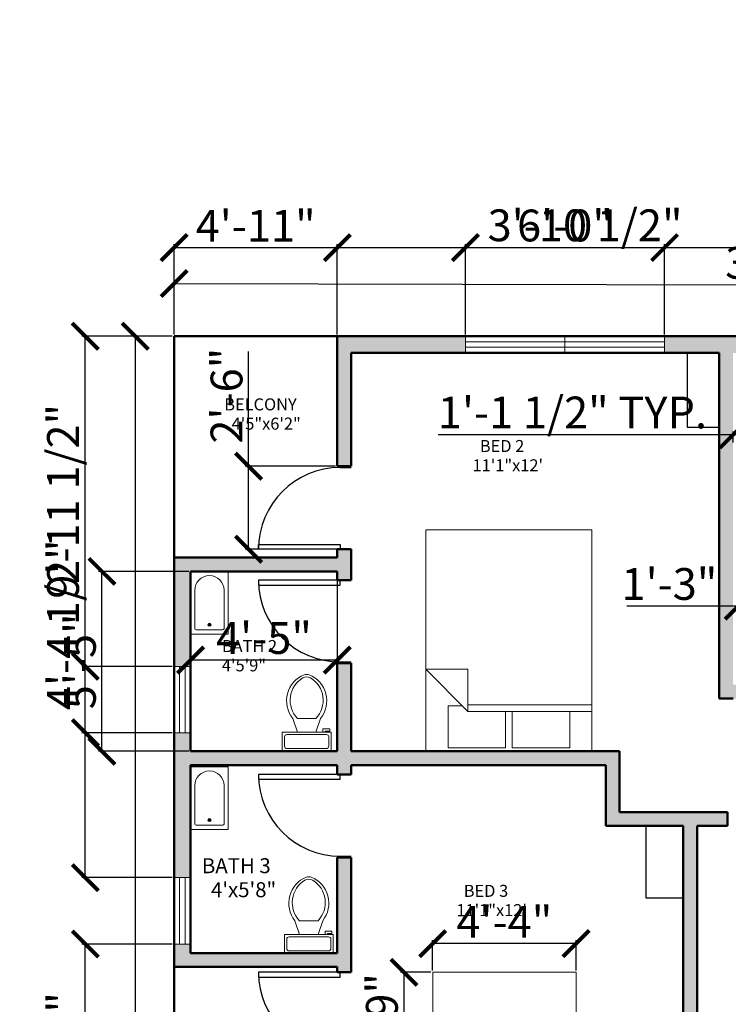
# Model space of a CAD drawing. Units: inches. Extents: x 3147 to 3847, y 1414 to 2207.
# Tile 6 of 7: x 3294 to 3550, y 1852 to 2207. Entities that reach past the tile are written whole.
import ezdxf

# ---------------------------------------------------------------- set-up
doc = ezdxf.new("R2010")
doc.units = ezdxf.units.IN
for name, color, linetype, lineweight in [('A-ANNO-DIMS', 2, 'Continuous', 18), ('A-AREA-IDEN', 7, 'Continuous', 18), ('A-DOOR', 3, 'Continuous', 25), ('A-FLOR-CASE', 32, 'Continuous', 25), ('A-FLOR-FIXT', 9, 'Continuous', 18), ('A-FURN', 8, 'Continuous', 18), ('A-GLAZ', 4, 'Continuous', 18), ('A-WALL', 7, 'Continuous', 50)]:
    doc.layers.add(name, color=color, linetype=linetype, lineweight=lineweight)
doc.layers.add('A-WALL-PATT', color=18, linetype='Continuous', lineweight=13, true_color=0x000000)
doc.styles.get("Standard").update_dxf_attribs({"font": 'arial.ttf'})
doc.dimstyles.new('ISO-25', dxfattribs={"dimtxt": 11.5, "dimasz": 9.5, "dimexe": 1.25, "dimexo": 0.625, "dimtad": 1, "dimdec": 0, "dimlunit": 3, "dimtxsty": 'Standard', "dimblk": 'ARCHTICK', "dimcen": 2.5, "dimadec": 0, "dimazin": 0, "dimtfac": 1, "dimtdec": 0, "dimtmove": 0, "dimatfit": 3, "dimfxl": 1, "dimarcsym": 0})

# ---------------------------------------------------------------- blocks, each defined once
blk = doc.blocks.new('*U4')
for p, q in [((-750, 0), (-750, -100)), ((0, 0), (0, -100))]:
    blk.add_line(p, q)
blk.add_lwpolyline([(0, 0), (0, 750), (-43.75, 750), (-43.75, 0)], close=True)
blk.add_arc((0, 0), 750, 90, 180)
blk = doc.blocks.new('*U3')
for p, q in [((0, 0), (0, -100)), ((750, 0), (750, -100))]:
    blk.add_line(p, q)
blk.add_lwpolyline([(0, 0), (0, 750), (43.75, 750), (43.75, 0)], close=True)
blk.add_arc((0, 0), 750, 0, 90)
blk = doc.blocks.new('Bath Tub - 26 x 60 in.')
for p, q in [((8, -18), (10, -18)), ((9, -17), (9, -19))]:
    blk.add_line(p, q)
blk.add_lwpolyline([(0, -36), (0, 0), (60, 0), (60, -36)], close=True)
for points in [[(4, -30), (4, -6)], [(6, -4), (42, -4)], [(42, -32), (6, -32)]]:
    blk.add_lwpolyline(points)
for radius in [1.5, 1]:
    blk.add_circle((9, -18), radius)
for centre, radius, start, end in [((5.75, -5.75), 1.77, 81.8699, 188.1301), ((42, -18), 14, 270, 90), ((5.75, -30.25), 1.77, 171.8699, 278.1301)]:
    blk.add_arc(centre, radius, start, end)
blk = doc.blocks.new('Toilet - top')
for p, q in [((9.5, -6), (9.5, -2)), ((-10, -8.5), (-8, -8.5)), ((-10, -9.5), (-10, -8.5)), ((-8, -8.5), (-8, -8)), ((-7, -8), (-7, -9.5)), ((-4, -8), (-6, -14)), ((4, -8), (6, -14)), ((-7, -9.5), (-10, -9.5)), ((4, -14), (-4, -14))]:
    blk.add_line(p, q)
blk.add_lwpolyline([(10.5, -8), (10.5, 0), (-10.5, 0), (-10.5, -8)], close=True)
for points in [[(-9.5, -2), (-9.5, -6)], [(8.5, -1), (-8.5, -1)], [(-8.5, -7), (8.5, -7)]]:
    blk.add_lwpolyline(points)
for centre, radius, start, end in [((-8.62, -1.88), 0.884, 81.8699, 188.1301), ((8.62, -1.88), 0.884, 351.8699, 98.1301), ((-8.62, -6.12), 0.884, 171.8699, 278.1301), ((8.62, -6.12), 0.884, 261.8699, 8.1301), ((3.52, -21.58), 12.17, 141.4691, 247.9714), ((4.2, -21.82), 11.33, 136.3677, 238.9468), ((-3.52, -21.58), 12.17, 292.0284, 38.5307), ((-4.2, -21.82), 11.33, 301.053, 43.6321), ((0, -27.88), 4, 245.7318, 294.2682), ((0, -29), 4, 254.8605, 285.1395)]:
    blk.add_arc(centre, radius, start, end)
blk = doc.blocks.new('Bed - Queen')
for p, q in [((0, -80.00003), (0, 0)), ((0, 0), (59.99999, 0)), ((59.99999, 0), (59.99999, -80.00003)), ((7.99999, -1.2), (28.79998, -1.2)), ((7.99999, -14.4), (7.99999, -1.2)), ((28.79998, -1.2), (28.79998, -14.4)), ((31.19999, -1.2), (51.99999, -1.2)), ((31.19999, -14.4), (31.19999, -1.2)), ((51.99999, -1.2), (51.99999, -16.4)), ((0, -14.4), (44.8, -14.4)), ((44.8, -16.8), (0, -16.8)), ((59.99999, -29.6), (44.8, -14.4)), ((44.8, -14.4), (44.8, -29.6)), ((51.99999, -16.4), (46.79936, -16.4)), ((44.8, -29.6), (59.99999, -29.6)), ((59.99999, -80.00003), (0, -80.00003))]:
    blk.add_line(p, q)
blk = doc.blocks.new('_ArchTick')
at = {"color": 0, "linetype": 'ByBlock', "const_width": 0.15}
blk.add_lwpolyline([(-0.5, -0.5), (0.5, 0.5)], dxfattribs=at)
blk = doc.blocks.new('*D22')
at = {"layer": 'A-ANNO-DIMS', "color": 0, "lineweight": -2, "transparency": 16777216}
for p, q in [((3349.14, 2093.05), (3334.5, 2093.05)), ((3335.75, 2093.05), (3335.75, 1495.05)), ((3349.14, 1495.05), (3334.5, 1495.05))]:
    blk.add_line(p, q, dxfattribs=at)
at = {"layer": 'Defpoints', "color": 0, "transparency": 16777216}
for p in [(3349.76, 2093.05), (3335.75, 1495.05), (3349.76, 1495.05)]:
    blk.add_point(p, dxfattribs=at)
at = {"layer": 'A-ANNO-DIMS', "color": 0, "lineweight": -2, "transparency": 16777216, "xscale": 9.5, "yscale": 9.5, "zscale": 9.5}
for p, rotation in [((3335.75, 2093.05), 90), ((3335.75, 1495.05), 270)]:
    blk.add_blockref('_ArchTick', p, dxfattribs=dict(at, rotation=rotation))
at = {"layer": 'A-ANNO-DIMS', "color": 0, "transparency": 16777216, "insert": (3329.25, 1794.05), "char_height": 11.5, "attachment_point": 5, "rotation": 90}
blk.add_mtext('49\'-10"', dxfattribs=at)
blk = doc.blocks.new('*D23')
at = {"layer": 'A-ANNO-DIMS', "color": 0, "lineweight": -2, "transparency": 16777216}
for p, q in [((3349.77, 2094.75), (3349.81, 2113.37)), ((3349.81, 2112.12), (3769.81, 2111.04)), ((3769.77, 2093.67), (3769.81, 2112.29))]:
    blk.add_line(p, q, dxfattribs=at)
at = {"layer": 'Defpoints', "color": 0, "transparency": 16777216}
for p in [(3769.81, 2111.04), (3349.76, 2094.13), (3769.76, 2093.05)]:
    blk.add_point(p, dxfattribs=at)
at = {"layer": 'A-ANNO-DIMS', "color": 0, "lineweight": -2, "transparency": 16777216, "xscale": 9.5, "yscale": 9.5, "zscale": 9.5}
for p, rotation in [((3349.81, 2112.12), 179.8528346034433), ((3769.81, 2111.04), 359.8528346034433)]:
    blk.add_blockref('_ArchTick', p, dxfattribs=dict(at, rotation=rotation))
at = {"layer": 'A-ANNO-DIMS', "color": 0, "transparency": 16777216, "insert": (3559.83, 2118.08), "char_height": 11.5, "attachment_point": 5, "rotation": 359.8528}
blk.add_mtext("35'", dxfattribs=at)
blk = doc.blocks.new('WIN-24IN')
for p, q in [((6, 24), (0, 24)), ((2, 0), (2, 24)), ((4, 0), (4, 24)), ((6, 0), (0, 0))]:
    blk.add_line(p, q)
blk = doc.blocks.new('*D29')
at = {"layer": 'A-ANNO-DIMS', "color": 0, "lineweight": -2, "transparency": 16777216}
for p, q in [((3568.76, 2054.03), (3568.76, 2207.49)), ((3565.99, 2054.03), (3570.01, 2054.03)), ((3568.76, 2031.36), (3568.76, 2054.03)), ((3565.99, 2031.36), (3570.01, 2031.36))]:
    blk.add_line(p, q, dxfattribs=at)
at = {"layer": 'Defpoints', "color": 0, "transparency": 16777216}
for p in [(3565.36, 2054.03), (3568.76, 2054.03), (3565.36, 2031.36)]:
    blk.add_point(p, dxfattribs=at)
at = {"layer": 'A-ANNO-DIMS', "color": 0, "lineweight": -2, "transparency": 16777216, "xscale": 9.5, "yscale": 9.5, "zscale": 9.5}
for p, rotation in [((3568.76, 2054.03), 90), ((3568.76, 2031.36), 270)]:
    blk.add_blockref('_ArchTick', p, dxfattribs=dict(at, rotation=rotation))
at = {"layer": 'A-ANNO-DIMS', "color": 0, "transparency": 16777216, "insert": (3562.19, 2135.51), "char_height": 11.5, "attachment_point": 5, "rotation": 90}
blk.add_mtext('TUB 1\'-10 1/2" TYP.', dxfattribs=at)
blk = doc.blocks.new('*D30')
at = {"layer": 'A-ANNO-DIMS', "color": 0, "lineweight": -2, "transparency": 16777216}
for p, q in [((3551.76, 2057.43), (3445.2, 2057.43)), ((3551.76, 2054.65), (3551.76, 2058.68)), ((3565.36, 2057.43), (3551.76, 2057.43)), ((3565.36, 2054.65), (3565.36, 2058.68))]:
    blk.add_line(p, q, dxfattribs=at)
at = {"layer": 'Defpoints', "color": 0, "transparency": 16777216}
for p in [(3551.76, 2057.43), (3551.76, 2054.03), (3565.36, 2054.03)]:
    blk.add_point(p, dxfattribs=at)
at = {"layer": 'A-ANNO-DIMS', "color": 0, "lineweight": -2, "transparency": 16777216, "xscale": 9.5, "yscale": 9.5, "zscale": 9.5, "rotation": 180}
blk.add_blockref('_ArchTick', (3551.76, 2057.43), dxfattribs=at)
at = {"layer": 'A-ANNO-DIMS', "color": 0, "lineweight": -2, "transparency": 16777216, "xscale": 9.5, "yscale": 9.5, "zscale": 9.5}
blk.add_blockref('_ArchTick', (3565.36, 2057.43), dxfattribs=at)
at = {"layer": 'A-ANNO-DIMS', "color": 0, "transparency": 16777216, "insert": (3493.73, 2064), "char_height": 11.5, "attachment_point": 5}
blk.add_mtext('1\'-1 1/2" TYP.', dxfattribs=at)
blk = doc.blocks.new('*D35')
at = {"layer": 'A-ANNO-DIMS', "color": 0, "lineweight": -2, "transparency": 16777216}
for p, q in [((3442.6, 1863.12), (3431.61, 1863.12)), ((3432.86, 1863.12), (3432.86, 1794.05)), ((3442.6, 1794.05), (3431.61, 1794.05))]:
    blk.add_line(p, q, dxfattribs=at)
at = {"layer": 'Defpoints', "color": 0, "transparency": 16777216}
for p in [(3443.22, 1863.12), (3432.86, 1794.05), (3443.22, 1794.05)]:
    blk.add_point(p, dxfattribs=at)
at = {"layer": 'A-ANNO-DIMS', "color": 0, "lineweight": -2, "transparency": 16777216, "xscale": 9.5, "yscale": 9.5, "zscale": 9.5}
for p, rotation in [((3432.86, 1863.12), 90), ((3432.86, 1794.05), 270)]:
    blk.add_blockref('_ArchTick', p, dxfattribs=dict(at, rotation=rotation))
at = {"layer": 'A-ANNO-DIMS', "color": 0, "transparency": 16777216, "insert": (3426.36, 1828.59), "char_height": 11.5, "attachment_point": 5, "rotation": 90}
blk.add_mtext('BED 5\'-9"', dxfattribs=at)
blk = doc.blocks.new('*D36')
at = {"layer": 'A-ANNO-DIMS', "color": 0, "lineweight": -2, "transparency": 16777216}
for p, q in [((3443.22, 1863.75), (3443.22, 1874.73)), ((3495.03, 1873.48), (3443.22, 1873.48)), ((3495.03, 1863.75), (3495.03, 1874.73))]:
    blk.add_line(p, q, dxfattribs=at)
at = {"layer": 'Defpoints', "color": 0, "transparency": 16777216}
for p in [(3443.22, 1873.48), (3443.22, 1863.12), (3495.03, 1863.12)]:
    blk.add_point(p, dxfattribs=at)
at = {"layer": 'A-ANNO-DIMS', "color": 0, "lineweight": -2, "transparency": 16777216, "xscale": 9.5, "yscale": 9.5, "zscale": 9.5, "rotation": 180}
blk.add_blockref('_ArchTick', (3443.22, 1873.48), dxfattribs=at)
at = {"layer": 'A-ANNO-DIMS', "color": 0, "lineweight": -2, "transparency": 16777216, "xscale": 9.5, "yscale": 9.5, "zscale": 9.5}
blk.add_blockref('_ArchTick', (3495.03, 1873.48), dxfattribs=at)
at = {"layer": 'A-ANNO-DIMS', "color": 0, "transparency": 16777216, "insert": (3469.12, 1879.86), "char_height": 11.5, "attachment_point": 5}
blk.add_mtext('4\'-4"', dxfattribs=at)
blk = doc.blocks.new('*D47')
at = {"layer": 'A-ANNO-DIMS', "color": 0, "lineweight": -2, "transparency": 16777216}
for p, q in [((3571.89, 1992.16), (3571.89, 2111.11)), ((3569.17, 1992.16), (3573.14, 1992.16)), ((3571.89, 1969.81), (3571.89, 1992.16)), ((3569.17, 1969.81), (3573.14, 1969.81))]:
    blk.add_line(p, q, dxfattribs=at)
at = {"layer": 'Defpoints', "color": 0, "transparency": 16777216}
for p in [(3568.54, 1992.16), (3571.89, 1992.16), (3568.54, 1969.81)]:
    blk.add_point(p, dxfattribs=at)
at = {"layer": 'A-ANNO-DIMS', "color": 0, "lineweight": -2, "transparency": 16777216, "xscale": 9.5, "yscale": 9.5, "zscale": 9.5}
for p, rotation in [((3571.89, 1992.16), 90), ((3571.89, 1969.81), 270)]:
    blk.add_blockref('_ArchTick', p, dxfattribs=dict(at, rotation=rotation))
at = {"layer": 'A-ANNO-DIMS', "color": 0, "transparency": 16777216, "insert": (3565.32, 2056.38), "char_height": 11.5, "attachment_point": 5, "rotation": 90}
blk.add_mtext('SINK 1\'-10 1/2"', dxfattribs=at)
blk = doc.blocks.new('*D48')
at = {"layer": 'A-ANNO-DIMS', "color": 0, "lineweight": -2, "transparency": 16777216}
for p, q in [((3553.64, 1995.51), (3513.41, 1995.51)), ((3553.64, 1992.78), (3553.64, 1996.76)), ((3568.54, 1995.51), (3553.64, 1995.51)), ((3568.54, 1992.78), (3568.54, 1996.76))]:
    blk.add_line(p, q, dxfattribs=at)
at = {"layer": 'Defpoints', "color": 0, "transparency": 16777216}
for p in [(3553.64, 1995.51), (3553.64, 1992.16), (3568.54, 1992.16)]:
    blk.add_point(p, dxfattribs=at)
at = {"layer": 'A-ANNO-DIMS', "color": 0, "lineweight": -2, "transparency": 16777216, "xscale": 9.5, "yscale": 9.5, "zscale": 9.5, "rotation": 180}
blk.add_blockref('_ArchTick', (3553.64, 1995.51), dxfattribs=at)
at = {"layer": 'A-ANNO-DIMS', "color": 0, "lineweight": -2, "transparency": 16777216, "xscale": 9.5, "yscale": 9.5, "zscale": 9.5}
blk.add_blockref('_ArchTick', (3568.54, 1995.51), dxfattribs=at)
at = {"layer": 'A-ANNO-DIMS', "color": 0, "transparency": 16777216, "insert": (3528.78, 2002.01), "char_height": 11.5, "attachment_point": 5}
blk.add_mtext('1\'-3"', dxfattribs=at)
blk = doc.blocks.new('*D62')
at = {"layer": 'A-ANNO-DIMS', "color": 0, "lineweight": -2, "transparency": 16777216}
for p, q in [((3349.76, 2093.67), (3349.76, 2126.35)), ((3349.76, 2125.1), (3408.76, 2125.1)), ((3408.76, 2093.67), (3408.76, 2126.35))]:
    blk.add_line(p, q, dxfattribs=at)
at = {"layer": 'Defpoints', "color": 0, "transparency": 16777216}
for p in [(3408.76, 2125.1), (3349.76, 2093.05), (3408.76, 2093.05)]:
    blk.add_point(p, dxfattribs=at)
at = {"layer": 'A-ANNO-DIMS', "color": 0, "lineweight": -2, "transparency": 16777216, "xscale": 9.5, "yscale": 9.5, "zscale": 9.5, "rotation": 180}
blk.add_blockref('_ArchTick', (3349.76, 2125.1), dxfattribs=at)
at = {"layer": 'A-ANNO-DIMS', "color": 0, "lineweight": -2, "transparency": 16777216, "xscale": 9.5, "yscale": 9.5, "zscale": 9.5}
blk.add_blockref('_ArchTick', (3408.76, 2125.1), dxfattribs=at)
at = {"layer": 'A-ANNO-DIMS', "color": 0, "transparency": 16777216, "insert": (3379.26, 2131.5), "char_height": 11.5, "attachment_point": 5}
blk.add_mtext('4\'-11"', dxfattribs=at)
blk = doc.blocks.new('*D63')
at = {"layer": 'A-ANNO-DIMS', "color": 0, "lineweight": -2, "transparency": 16777216}
for p, q in [((3408.76, 2093.67), (3408.76, 2126.35)), ((3408.76, 2125.1), (3455.03, 2125.1)), ((3455.03, 2093.67), (3455.03, 2126.35)), ((3455.03, 2125.1), (3532.08, 2125.1))]:
    blk.add_line(p, q, dxfattribs=at)
at = {"layer": 'Defpoints', "color": 0, "transparency": 16777216}
for p in [(3455.03, 2125.1), (3408.76, 2093.05), (3455.03, 2093.05)]:
    blk.add_point(p, dxfattribs=at)
at = {"layer": 'A-ANNO-DIMS', "color": 0, "lineweight": -2, "transparency": 16777216, "xscale": 9.5, "yscale": 9.5, "zscale": 9.5, "rotation": 180}
blk.add_blockref('_ArchTick', (3408.76, 2125.1), dxfattribs=at)
at = {"layer": 'A-ANNO-DIMS', "color": 0, "lineweight": -2, "transparency": 16777216, "xscale": 9.5, "yscale": 9.5, "zscale": 9.5}
blk.add_blockref('_ArchTick', (3455.03, 2125.1), dxfattribs=at)
at = {"layer": 'A-ANNO-DIMS', "color": 0, "transparency": 16777216, "insert": (3498.3, 2131.67), "char_height": 11.5, "attachment_point": 5}
blk.add_mtext('3\'-10 1/2"', dxfattribs=at)
blk = doc.blocks.new('*D64')
at = {"layer": 'A-ANNO-DIMS', "color": 0, "lineweight": -2, "transparency": 16777216}
for p, q in [((3455.03, 2093.67), (3455.03, 2126.35)), ((3455.03, 2125.1), (3527.03, 2125.1)), ((3527.03, 2093.67), (3527.03, 2126.35))]:
    blk.add_line(p, q, dxfattribs=at)
at = {"layer": 'Defpoints', "color": 0, "transparency": 16777216}
for p in [(3527.03, 2125.1), (3455.03, 2093.05), (3527.03, 2093.05)]:
    blk.add_point(p, dxfattribs=at)
at = {"layer": 'A-ANNO-DIMS', "color": 0, "lineweight": -2, "transparency": 16777216, "xscale": 9.5, "yscale": 9.5, "zscale": 9.5, "rotation": 180}
blk.add_blockref('_ArchTick', (3455.03, 2125.1), dxfattribs=at)
at = {"layer": 'A-ANNO-DIMS', "color": 0, "lineweight": -2, "transparency": 16777216, "xscale": 9.5, "yscale": 9.5, "zscale": 9.5}
blk.add_blockref('_ArchTick', (3527.03, 2125.1), dxfattribs=at)
at = {"layer": 'A-ANNO-DIMS', "color": 0, "transparency": 16777216, "insert": (3491.03, 2131.6), "char_height": 11.5, "attachment_point": 5}
blk.add_mtext('6\'-0"', dxfattribs=at)
blk = doc.blocks.new('*D65')
at = {"layer": 'A-ANNO-DIMS', "color": 0, "lineweight": -2, "transparency": 16777216}
for p, q in [((3527.03, 2093.67), (3527.03, 2126.35)), ((3527.03, 2125.1), (3576.44, 2125.1)), ((3576.44, 2093.67), (3576.44, 2126.35)), ((3576.44, 2125.1), (3645.01, 2125.1))]:
    blk.add_line(p, q, dxfattribs=at)
at = {"layer": 'Defpoints', "color": 0, "transparency": 16777216}
for p in [(3576.44, 2125.1), (3527.03, 2093.05), (3576.44, 2093.05)]:
    blk.add_point(p, dxfattribs=at)
at = {"layer": 'A-ANNO-DIMS', "color": 0, "lineweight": -2, "transparency": 16777216, "xscale": 9.5, "yscale": 9.5, "zscale": 9.5, "rotation": 180}
blk.add_blockref('_ArchTick', (3527.03, 2125.1), dxfattribs=at)
at = {"layer": 'A-ANNO-DIMS', "color": 0, "lineweight": -2, "transparency": 16777216, "xscale": 9.5, "yscale": 9.5, "zscale": 9.5}
blk.add_blockref('_ArchTick', (3576.44, 2125.1), dxfattribs=at)
at = {"layer": 'A-ANNO-DIMS', "color": 0, "transparency": 16777216, "insert": (3615.48, 2131.67), "char_height": 11.5, "attachment_point": 5}
blk.add_mtext('4\'-1 1/2"', dxfattribs=at)
blk = doc.blocks.new('*D80')
at = {"layer": 'A-ANNO-DIMS', "color": 0, "lineweight": -2, "transparency": 16777216}
for p, q in [((3349.14, 1873.34), (3316.46, 1873.34)), ((3317.71, 1776.88), (3317.71, 1873.34)), ((3349.14, 1776.88), (3316.46, 1776.88))]:
    blk.add_line(p, q, dxfattribs=at)
at = {"layer": 'Defpoints', "color": 0, "transparency": 16777216}
for p in [(3317.71, 1873.34), (3349.76, 1873.34), (3349.76, 1776.88)]:
    blk.add_point(p, dxfattribs=at)
at = {"layer": 'A-ANNO-DIMS', "color": 0, "lineweight": -2, "transparency": 16777216, "xscale": 9.5, "yscale": 9.5, "zscale": 9.5}
for p, rotation in [((3317.71, 1873.34), 90), ((3317.71, 1776.88), 270)]:
    blk.add_blockref('_ArchTick', p, dxfattribs=dict(at, rotation=rotation))
at = {"layer": 'A-ANNO-DIMS', "color": 0, "transparency": 16777216, "insert": (3311.14, 1825.11), "char_height": 11.5, "attachment_point": 5, "rotation": 90}
blk.add_mtext('8\'-0 1/2"', dxfattribs=at)
blk = doc.blocks.new('*D81')
at = {"layer": 'A-ANNO-DIMS', "color": 0, "lineweight": -2, "transparency": 16777216}
for p, q in [((3317.71, 1949.71), (3317.71, 2018.29)), ((3349.14, 1949.71), (3316.46, 1949.71)), ((3317.71, 1897.34), (3317.71, 1949.71)), ((3349.14, 1897.34), (3316.46, 1897.34))]:
    blk.add_line(p, q, dxfattribs=at)
at = {"layer": 'Defpoints', "color": 0, "transparency": 16777216}
for p in [(3317.71, 1949.71), (3349.76, 1949.71), (3349.76, 1897.34)]:
    blk.add_point(p, dxfattribs=at)
at = {"layer": 'A-ANNO-DIMS', "color": 0, "lineweight": -2, "transparency": 16777216, "xscale": 9.5, "yscale": 9.5, "zscale": 9.5}
for p, rotation in [((3317.71, 1949.71), 90), ((3317.71, 1897.34), 270)]:
    blk.add_blockref('_ArchTick', p, dxfattribs=dict(at, rotation=rotation))
at = {"layer": 'A-ANNO-DIMS', "color": 0, "transparency": 16777216, "insert": (3311.14, 1988.75), "char_height": 11.5, "attachment_point": 5, "rotation": 90}
blk.add_mtext('4\'-4 1/2"', dxfattribs=at)
blk = doc.blocks.new('*D82')
at = {"layer": 'A-ANNO-DIMS', "color": 0, "lineweight": -2, "transparency": 16777216}
for p, q in [((3349.14, 2093.05), (3316.46, 2093.05)), ((3317.71, 1973.71), (3317.71, 2093.05)), ((3349.14, 1973.71), (3316.46, 1973.71))]:
    blk.add_line(p, q, dxfattribs=at)
at = {"layer": 'Defpoints', "color": 0, "transparency": 16777216}
for p in [(3317.71, 2093.05), (3349.76, 2093.05), (3349.76, 1973.71)]:
    blk.add_point(p, dxfattribs=at)
at = {"layer": 'A-ANNO-DIMS', "color": 0, "lineweight": -2, "transparency": 16777216, "xscale": 9.5, "yscale": 9.5, "zscale": 9.5}
for p, rotation in [((3317.71, 2093.05), 90), ((3317.71, 1973.71), 270)]:
    blk.add_blockref('_ArchTick', p, dxfattribs=dict(at, rotation=rotation))
at = {"layer": 'A-ANNO-DIMS', "color": 0, "transparency": 16777216, "insert": (3311.14, 2033.38), "char_height": 11.5, "attachment_point": 5, "rotation": 90}
blk.add_mtext('9\'-11 1/2"', dxfattribs=at)
blk = doc.blocks.new('*D83')
at = {"layer": 'A-ANNO-DIMS', "color": 0, "lineweight": -2, "transparency": 16777216}
for p, q in [((3376.71, 2046.06), (3376.71, 2087.58)), ((3408.14, 2046.06), (3375.46, 2046.06)), ((3376.71, 2016.06), (3376.71, 2046.06)), ((3408.14, 2016.06), (3375.46, 2016.06))]:
    blk.add_line(p, q, dxfattribs=at)
at = {"layer": 'Defpoints', "color": 0, "transparency": 16777216}
for p in [(3376.71, 2046.06), (3408.76, 2046.06), (3408.76, 2016.06)]:
    blk.add_point(p, dxfattribs=at)
at = {"layer": 'A-ANNO-DIMS', "color": 0, "lineweight": -2, "transparency": 16777216, "xscale": 9.5, "yscale": 9.5, "zscale": 9.5}
for p, rotation in [((3376.71, 2046.06), 90), ((3376.71, 2016.06), 270)]:
    blk.add_blockref('_ArchTick', p, dxfattribs=dict(at, rotation=rotation))
at = {"layer": 'A-ANNO-DIMS', "color": 0, "transparency": 16777216, "insert": (3370.22, 2071.57), "char_height": 11.5, "attachment_point": 5, "rotation": 90}
blk.add_mtext('2\'-6"', dxfattribs=at)
blk = doc.blocks.new('*D86')
at = {"layer": 'A-ANNO-DIMS', "color": 0, "lineweight": -2, "transparency": 16777216}
for p, q in [((3355.14, 2008.05), (3322.46, 2008.05)), ((3323.71, 1943.05), (3323.71, 2008.05)), ((3355.14, 1943.05), (3322.46, 1943.05))]:
    blk.add_line(p, q, dxfattribs=at)
at = {"layer": 'Defpoints', "color": 0, "transparency": 16777216}
for p in [(3323.71, 2008.05), (3355.76, 2008.05), (3355.76, 1943.05)]:
    blk.add_point(p, dxfattribs=at)
at = {"layer": 'A-ANNO-DIMS', "color": 0, "lineweight": -2, "transparency": 16777216, "xscale": 9.5, "yscale": 9.5, "zscale": 9.5}
for p, rotation in [((3323.71, 2008.05), 90), ((3323.71, 1943.05), 270)]:
    blk.add_blockref('_ArchTick', p, dxfattribs=dict(at, rotation=rotation))
at = {"layer": 'A-ANNO-DIMS', "color": 0, "transparency": 16777216, "insert": (3317.24, 1975.55), "char_height": 11.5, "attachment_point": 5, "rotation": 90}
blk.add_mtext('5\'-5"', dxfattribs=at)
blk = doc.blocks.new('*D87')
at = {"layer": 'A-ANNO-DIMS', "color": 0, "lineweight": -2, "transparency": 16777216}
for p, q in [((3355.76, 2007.42), (3355.76, 1974.75)), ((3408.76, 2007.42), (3408.76, 1974.75)), ((3408.76, 1976), (3355.76, 1976))]:
    blk.add_line(p, q, dxfattribs=at)
at = {"layer": 'Defpoints', "color": 0, "transparency": 16777216}
for p in [(3355.76, 2008.05), (3408.76, 2008.05), (3355.76, 1976)]:
    blk.add_point(p, dxfattribs=at)
at = {"layer": 'A-ANNO-DIMS', "color": 0, "lineweight": -2, "transparency": 16777216, "xscale": 9.5, "yscale": 9.5, "zscale": 9.5}
for p, rotation in [((3355.76, 1976), 179.9999999999992), ((3408.76, 1976), 359.9999999999992)]:
    blk.add_blockref('_ArchTick', p, dxfattribs=dict(at, rotation=rotation))
at = {"layer": 'A-ANNO-DIMS', "color": 0, "transparency": 16777216, "insert": (3382.26, 1982.47), "char_height": 11.5, "attachment_point": 5}
blk.add_mtext('4\'-5"', dxfattribs=at)

msp = doc.modelspace()

# ---------------------------------------------------------------- hatches: boundary and pattern name
at = {"layer": 'A-WALL-PATT'}
h = msp.add_hatch(color=256, dxfattribs=at)
h.dxf.hatch_style = 1
h.paths.add_polyline_path([(3616.76, 2093.05), (3594.02, 2093.05), (3594.02, 2087.05), (3611.76, 2087.05), (3611.76, 1993.05), (3616.76, 1993.05), (3628.76, 1993.05), (3628.76, 1996.99), (3628.76, 1998.05), (3616.76, 1998.05), (3616.76, 2087.05)])
h.paths.add_polyline_path([(3576.44, 2093.05), (3527.03, 2093.05), (3527.03, 2087.05), (3546.76, 2087.05), (3546.76, 1962.05), (3551.76, 1962.05), (3590.76, 1962.05), (3590.76, 1921.05), (3585.76, 1921.05), (3585.76, 1916.05), (3590.76, 1916.05), (3590.76, 1895.05), (3595.76, 1895.05), (3595.76, 1962.05), (3611.76, 1962.05), (3616.76, 1962.05), (3616.76, 1969.05), (3611.76, 1969.05), (3611.76, 1967.05), (3551.76, 1967.05), (3551.76, 2087.05), (3576.44, 2087.05)])
h.paths.add_polyline_path([(3455.03, 2093.05), (3408.76, 2093.05), (3408.76, 2087.05), (3408.76, 2046.06), (3413.76, 2046.06), (3413.76, 2087.05), (3455.03, 2087.05)])
h.paths.add_polyline_path([(3355.76, 2008.05), (3408.76, 2008.05), (3408.76, 2004.83), (3413.76, 2004.83), (3413.76, 2008.05), (3413.76, 2013.05), (3413.76, 2016.06), (3408.76, 2016.06), (3408.76, 2013.05), (3355.76, 2013.05), (3349.76, 2013.05), (3349.76, 1973.71), (3355.76, 1973.71)])
h.paths.add_polyline_path([(3413.76, 1974.83), (3408.76, 1974.83), (3408.76, 1943.05), (3355.76, 1943.05), (3355.76, 1949.71), (3349.76, 1949.71), (3349.76, 1897.34), (3355.76, 1897.34), (3355.76, 1938.05), (3408.76, 1938.05), (3408.76, 1934.63), (3413.76, 1934.63), (3413.76, 1938.05), (3505.76, 1938.05), (3505.76, 1916.05), (3533.76, 1916.05), (3533.76, 1904.63), (3533.76, 1831.83), (3538.76, 1831.83), (3538.76, 1904.63), (3538.76, 1916.05), (3546.76, 1916.05), (3549.76, 1916.05), (3549.76, 1921.05), (3546.76, 1921.05), (3510.76, 1921.05), (3510.76, 1938.05), (3510.76, 1943.05), (3413.76, 1943.05)])
h.paths.add_polyline_path([(3413.76, 1904.63), (3408.76, 1904.63), (3408.76, 1870.05), (3355.76, 1870.05), (3355.76, 1873.34), (3349.76, 1873.34), (3349.76, 1865.05), (3355.76, 1865.05), (3408.76, 1865.05), (3408.76, 1863.11), (3409.83, 1863.11), (3413.76, 1863.11)], flags=17)
h.paths.add_polyline_path([(3538.76, 1795.83), (3533.76, 1795.83), (3533.76, 1794.05), (3413.76, 1794.05), (3413.76, 1833.11), (3408.76, 1833.11), (3408.76, 1794.05), (3355.76, 1794.05), (3349.76, 1794.05), (3349.76, 1776.88), (3355.76, 1776.88), (3355.76, 1789.05), (3413.76, 1789.05), (3475.76, 1789.05), (3475.76, 1731.91), (3480.76, 1731.91), (3480.76, 1789.05), (3538.76, 1789.05)])
h.paths.add_polyline_path([(3432.14, 1733.05), (3413.76, 1733.05), (3355.76, 1733.05), (3355.76, 1740.88), (3349.76, 1740.88), (3349.76, 1720.47), (3355.76, 1720.47), (3355.76, 1729.05), (3413.76, 1729.05), (3432.14, 1729.05)])
h.paths.add_polyline_path([(3480.76, 1695.91), (3476.83, 1695.91), (3475.76, 1695.91), (3475.76, 1693.05), (3413.76, 1693.05), (3355.76, 1693.05), (3355.76, 1696.47), (3349.76, 1696.47), (3349.76, 1671.27), (3355.76, 1671.27), (3355.76, 1688.05), (3413.76, 1688.05), (3415.76, 1688.05), (3415.76, 1673.71), (3420.76, 1673.71), (3420.76, 1688.05), (3480.76, 1688.05)])
h.paths.add_polyline_path([(3420.76, 1643.71), (3415.76, 1643.71), (3415.76, 1642.05), (3413.76, 1642.05), (3355.76, 1642.05), (3355.76, 1647.27), (3349.76, 1647.27), (3349.76, 1598.35), (3355.76, 1598.35), (3355.76, 1637.05), (3401.76, 1637.05), (3401.76, 1634.26), (3406.76, 1634.26), (3406.76, 1637.05), (3413.76, 1637.05), (3420.76, 1637.05)])
h.paths.add_polyline_path([(3406.76, 1604.26), (3401.76, 1604.26), (3401.76, 1572.05), (3355.76, 1572.05), (3355.76, 1574.35), (3349.76, 1574.35), (3349.76, 1553.05), (3349.76, 1495.05), (3371.89, 1495.05), (3371.89, 1501.05), (3355.76, 1501.05), (3355.76, 1559.05), (3355.76, 1567.05), (3406.76, 1567.05), (3406.76, 1572.05)])
h.paths.add_polyline_path([(3534.41, 1501.05), (3419.89, 1501.05), (3419.89, 1495.05), (3534.41, 1495.05)])
h.paths.add_polyline_path([(3769.76, 1509.48), (3763.76, 1509.48), (3763.76, 1501.05), (3600.76, 1501.05), (3600.76, 1548.51), (3595.76, 1548.51), (3595.76, 1501.05), (3582.41, 1501.05), (3582.41, 1495.05), (3769.76, 1495.05)])
h.paths.add_polyline_path([(3769.76, 1645.82), (3763.76, 1645.82), (3763.76, 1593.05), (3664.76, 1593.05), (3619.76, 1593.05), (3619.76, 1674.05), (3614.76, 1674.05), (3614.76, 1593.05), (3595.76, 1593.05), (3595.76, 1584.51), (3600.76, 1584.51), (3600.76, 1588.05), (3619.76, 1588.05), (3664.76, 1588.05), (3763.76, 1588.05), (3763.76, 1569.48), (3769.76, 1569.48)])
h.paths.add_polyline_path([(3769.76, 1731.24), (3763.76, 1731.24), (3763.76, 1718.05), (3664.76, 1718.05), (3595.76, 1718.05), (3595.76, 1723.05), (3590.76, 1723.05), (3590.76, 1713.05), (3595.76, 1713.05), (3614.76, 1713.05), (3614.76, 1710.05), (3619.76, 1710.05), (3619.76, 1713.05), (3664.76, 1713.05), (3763.76, 1713.05), (3763.76, 1693.82), (3769.76, 1693.82)])
h.paths.add_polyline_path([(3769.76, 1872.64), (3763.76, 1872.64), (3763.76, 1854.05), (3664.76, 1854.05), (3595.76, 1854.05), (3595.76, 1859.05), (3590.76, 1859.05), (3590.76, 1759.05), (3595.76, 1759.05), (3595.76, 1849.05), (3664.76, 1849.05), (3763.76, 1849.05), (3763.76, 1815.24), (3769.76, 1815.24)])
h.paths.add_polyline_path([(3769.76, 1998.05), (3763.76, 1998.05), (3763.76, 1968.64), (3769.76, 1968.64)])
h.paths.add_polyline_path([(3763.76, 1998.05), (3664.76, 1998.05), (3664.76, 1993.05), (3763.76, 1993.05)])

# ---------------------------------------------------------------- linework, layer by layer
at = {"layer": 'A-FLOR-CASE'}
for p, q in [((3535.16, 2087.05), (3535.16, 2060.23)), ((3535.16, 2060.23), (3546.76, 2060.23)), ((3520.2, 1916.05), (3520.2, 1889.99)), ((3520.2, 1889.99), (3533.76, 1889.99))]:
    msp.add_line(p, q, dxfattribs=at)
at = {"layer": 'A-GLAZ'}
for p, q in [((3455.03, 2087.05), (3455.03, 2093.05)), ((3491.03, 2087.05), (3491.03, 2093.05)), ((3527.03, 2087.05), (3527.03, 2093.05)), ((3455.03, 2091.05), (3527.03, 2091.05)), ((3455.03, 2089.05), (3527.03, 2089.05))]:
    msp.add_line(p, q, dxfattribs=at)
at = {"layer": 'A-WALL'}
for p, q in [((3349.76, 1553.05), (3349.76, 2093.05)), ((3349.76, 2093.05), (3769.76, 2093.05)), ((3408.76, 2087.05), (3408.76, 2093.05)), ((3408.76, 2046.06), (3408.76, 2087.05)), ((3413.76, 2087.05), (3546.76, 2087.05)), ((3413.76, 2046.06), (3413.76, 2087.05)), ((3546.76, 1962.05), (3546.76, 2087.05)), ((3408.76, 2046.06), (3413.76, 2046.06)), ((3408.76, 2013.05), (3408.76, 2016.06)), ((3408.76, 2016.06), (3413.76, 2016.06)), ((3413.76, 2013.05), (3413.76, 2016.06)), ((3355.76, 2013.05), (3349.76, 2013.05)), ((3355.76, 2013.05), (3408.76, 2013.05)), ((3413.76, 2013.05), (3413.76, 2008.05)), ((3355.76, 2008.05), (3408.76, 2008.05)), ((3355.76, 1943.05), (3355.76, 2008.05)), ((3408.76, 2004.83), (3408.76, 2008.05)), ((3413.76, 2004.83), (3413.76, 2008.05)), ((3408.76, 2004.83), (3413.76, 2004.83)), ((3408.76, 1974.83), (3413.76, 1974.83)), ((3408.76, 1943.05), (3408.76, 1974.83)), ((3413.76, 1943.05), (3413.76, 1974.83)), ((3551.76, 1962.05), (3546.76, 1962.05)), ((3355.76, 1943.05), (3408.76, 1943.05)), ((3413.76, 1943.05), (3510.76, 1943.05)), ((3510.76, 1938.05), (3510.76, 1943.05)), ((3355.76, 1938.05), (3408.76, 1938.05)), ((3355.76, 1870.05), (3355.76, 1938.05)), ((3408.76, 1934.63), (3408.76, 1938.05)), ((3413.76, 1938.05), (3505.76, 1938.05)), ((3413.76, 1934.63), (3413.76, 1938.05)), ((3505.76, 1938.05), (3505.76, 1916.05)), ((3510.76, 1938.05), (3510.76, 1921.05)), ((3408.76, 1934.63), (3413.76, 1934.63)), ((3510.76, 1921.05), (3546.76, 1921.05)), ((3546.76, 1921.05), (3549.76, 1921.05)), ((3549.76, 1921.05), (3549.76, 1916.05)), ((3505.76, 1916.05), (3533.76, 1916.05)), ((3538.76, 1916.05), (3546.76, 1916.05)), ((3546.76, 1916.05), (3549.76, 1916.05)), ((3408.76, 1904.63), (3413.76, 1904.63)), ((3408.76, 1870.05), (3408.76, 1904.63)), ((3413.76, 1863.11), (3413.76, 1904.63)), ((3355.76, 1870.05), (3408.76, 1870.05)), ((3355.76, 1865.05), (3349.76, 1865.05)), ((3355.76, 1865.05), (3408.76, 1865.05)), ((3408.76, 1863.11), (3408.76, 1865.05)), ((3408.76, 1863.11), (3408.76, 1865.05)), ((3408.76, 1863.11), (3413.76, 1863.11)), ((3413.76, 1863.11), (3413.76, 1865.05))]:
    msp.add_line(p, q, dxfattribs=at)
for points in [[(3533.76, 1831.83), (3533.76, 1904.63), (3533.76, 1916.05)], [(3538.76, 1831.83), (3538.76, 1904.63), (3538.76, 1916.05)]]:
    msp.add_lwpolyline(points, dxfattribs=at)

# ---------------------------------------------------------------- block references
at = {"layer": 'A-DOOR', "xscale": 0.0393700787401575, "yscale": 0.0393700787401575, "zscale": 0.0393700787401575, "rotation": 90}
for name, p in [('*U3', (3409.83, 2016.06)), ('*U4', (3409.83, 2004.83)), ('*U4', (3409.83, 1934.63)), ('*U4', (3409.83, 1863.11))]:
    msp.add_blockref(name, p, dxfattribs=at)
at = {"layer": 'A-FLOR-FIXT'}
for name, p, xscale, yscale, zscale, rotation in [('Bath Tub - 26 x 60 in.', (3355.76, 1985.38), 0.3777777777777778, 0.3777777777777778, 0.3777777777777778, 90), ('Toilet - top', (3397.69, 1943.18), 0.8374824719350153, 0.8374824719350153, 0.8374824719350153, 180), ('Bath Tub - 26 x 60 in.', (3355.76, 1914.76), 0.3777777777777778, 0.3777777777777778, 0.3777777777777778, 90), ('Toilet - top', (3398.46, 1870.05), 0.8374824719350153, 0.8374824719350153, 0.8374824719350153, 180)]:
    msp.add_blockref(name, p, dxfattribs=dict(at, xscale=xscale, yscale=yscale, zscale=zscale, rotation=rotation))
at = {"layer": 'A-FURN', "rotation": 180}
msp.add_blockref('Bed - Queen', (3500.77, 1943.05), dxfattribs=at)
at = {"layer": 'A-FURN', "xscale": 0.8634101176796084, "yscale": 0.8634101176796084, "zscale": 0.8634101176796084, "rotation": 180}
msp.add_blockref('Bed - Queen', (3495.03, 1794.05), dxfattribs=at)
at = {"layer": 'A-GLAZ'}
for p in [(3349.76, 1949.71), (3349.76, 1873.34)]:
    msp.add_blockref('WIN-24IN', p, dxfattribs=at)

# ---------------------------------------------------------------- texts
at = {"layer": 'A-AREA-IDEN'}
for s, height, p in [('BELCONY', 4.34, (3367.91, 2066.25)), ('  4\'5"x6\'2"', 4.3404, (3367.92, 2059.28)), ('  BED 2', 4.34, (3457.62, 2051.19)), ('11\'1"x12\'', 4.34, (3457.63, 2044.22)), ('BATH 2', 4.34, (3367.05, 1978.89)), ('4\'5\'9"', 4.34, (3367.06, 1971.91)), ('BATH 3', 5.408, (3359.83, 1898.94)), ('  4\'x5\'8"', 5.408, (3359.83, 1890.26)), ('  BED 3', 4.34, (3451.8, 1890.39)), ('11\'1"x12\'', 4.34, (3451.81, 1883.41))]:
    msp.add_text(s, height=height, rotation=0.0333, dxfattribs=at).set_placement(p)

# ---------------------------------------------------------------- dimensions: what is measured, and where the dimension line sits
at = {"layer": 'A-ANNO-DIMS'}
for base, p1, p2, angle, text, picture, middle in [((3568.76, 2054.03), (3565.36, 2031.36), (3565.36, 2054.03), 90, 'TUB <> TYP.', '*D29', (3562.19, 2135.51)), ((3571.894, 1992.1557), (3568.5419, 1969.8089), (3568.5419, 1992.1557), 90, 'SINK <>', '*D47', (3565.3229, 2056.3841)), ((3551.76, 2057.43), (3565.36, 2054.03), (3551.76, 2054.03), 180, '<> TYP.', '*D30', (3493.73, 2064)), ((3432.86, 1794.05), (3443.22, 1863.12), (3443.22, 1794.05), 270, 'BED <>', '*D35', (3426.36, 1828.59))]:
    dim = msp.add_linear_dim(base=base, p1=p1, p2=p2, angle=angle, text=text, dimstyle='ISO-25', override={"dimdec": 1, "dimlfac": 1, "dimrnd": 0, "dimzin": 1, "dimdsep": 46, "dimlunit": 4, "dimfrac": 2}, dxfattribs=at)
    dim.commit()
    dim.dimension.update_dxf_attribs({"geometry": picture, "text_midpoint": middle})
for base, p1, p2, picture, middle in [((3455.03, 2125.1), (3408.76, 2093.05), (3455.03, 2093.05), '*D63', (3498.3, 2131.67)), ((3576.44, 2125.1), (3527.03, 2093.05), (3576.44, 2093.05), '*D65', (3615.48, 2131.67)), ((3408.76, 2125.1), (3349.76, 2093.05), (3408.76, 2093.05), '*D62', (3379.26, 2131.5)), ((3527.03, 2125.1), (3455.03, 2093.05), (3527.03, 2093.05), '*D64', (3491.03, 2131.6))]:
    dim = msp.add_linear_dim(base=base, p1=p1, p2=p2, dimstyle='ISO-25', override={"dimdec": 1, "dimlfac": 1, "dimrnd": 0, "dimzin": 1, "dimdsep": 46, "dimlunit": 4, "dimfrac": 2}, dxfattribs=at)
    dim.commit()
    dim.dimension.update_dxf_attribs({"geometry": picture, "text_midpoint": middle})
dim = msp.add_aligned_dim(p1=(3349.76, 2094.13), p2=(3769.76, 2093.05), distance=17.99, dimstyle='ISO-25', override={"dimclrd": 0, "dimclre": 0, "dimclrt": 0}, dxfattribs=at)
dim.commit()
dim.dimension.update_dxf_attribs({"geometry": '*D23', "text_midpoint": (3559.83, 2118.08)})
for base, p1, p2, angle, override, picture, middle in [((3317.71, 2093.05), (3349.76, 1973.71), (3349.76, 2093.05), 90, {"dimdec": 1, "dimlfac": 1, "dimrnd": 0, "dimzin": 1, "dimdsep": 46, "dimlunit": 4, "dimfrac": 2}, '*D82', (3311.14, 2033.38)), ((3335.75, 1495.05), (3349.76, 2093.05), (3349.76, 1495.05), 90, {"dimclrd": 0, "dimclre": 0, "dimclrt": 0}, '*D22', (3329.25, 1794.05)), ((3376.71, 2046.06), (3408.76, 2016.06), (3408.76, 2046.06), 90, {"dimdec": 1, "dimlfac": 1, "dimrnd": 0, "dimzin": 1, "dimdsep": 46, "dimlunit": 4, "dimfrac": 2}, '*D83', (3370.22, 2071.57)), ((3317.71, 1949.71), (3349.76, 1897.34), (3349.76, 1949.71), 90, {"dimdec": 1, "dimlfac": 1, "dimrnd": 0, "dimzin": 1, "dimdsep": 46, "dimlunit": 4, "dimfrac": 2}, '*D81', (3311.14, 1988.75)), ((3323.71, 2008.05), (3355.76, 1943.05), (3355.76, 2008.05), 90, {"dimdec": 1, "dimlfac": 1, "dimrnd": 0, "dimzin": 1, "dimdsep": 46, "dimlunit": 4, "dimfrac": 2}, '*D86', (3317.24, 1975.55)), ((3355.76, 1976), (3408.76, 2008.05), (3355.76, 2008.05), 180, {"dimdec": 1, "dimlfac": 1, "dimrnd": 0, "dimzin": 1, "dimdsep": 46, "dimlunit": 4, "dimfrac": 2}, '*D87', (3382.26, 1982.47)), ((3553.64, 1995.51), (3568.54, 1992.16), (3553.64, 1992.16), 180, {"dimdec": 1, "dimlfac": 1, "dimrnd": 0, "dimzin": 1, "dimdsep": 46, "dimlunit": 4, "dimfrac": 2}, '*D48', (3528.78, 2002.01)), ((3443.22, 1873.48), (3495.03, 1863.12), (3443.22, 1863.12), 180, {"dimdec": 1, "dimlfac": 1, "dimrnd": 0, "dimzin": 1, "dimdsep": 46, "dimlunit": 4, "dimfrac": 2}, '*D36', (3469.12, 1879.86)), ((3317.71, 1873.34), (3349.76, 1776.88), (3349.76, 1873.34), 90, {"dimdec": 1, "dimlfac": 1, "dimrnd": 0, "dimzin": 1, "dimdsep": 46, "dimlunit": 4, "dimfrac": 2}, '*D80', (3311.14, 1825.11))]:
    dim = msp.add_linear_dim(base=base, p1=p1, p2=p2, angle=angle, dimstyle='ISO-25', override=override, dxfattribs=at)
    dim.commit()
    dim.dimension.update_dxf_attribs({"geometry": picture, "text_midpoint": middle})

doc.saveas('drawing.dxf')
